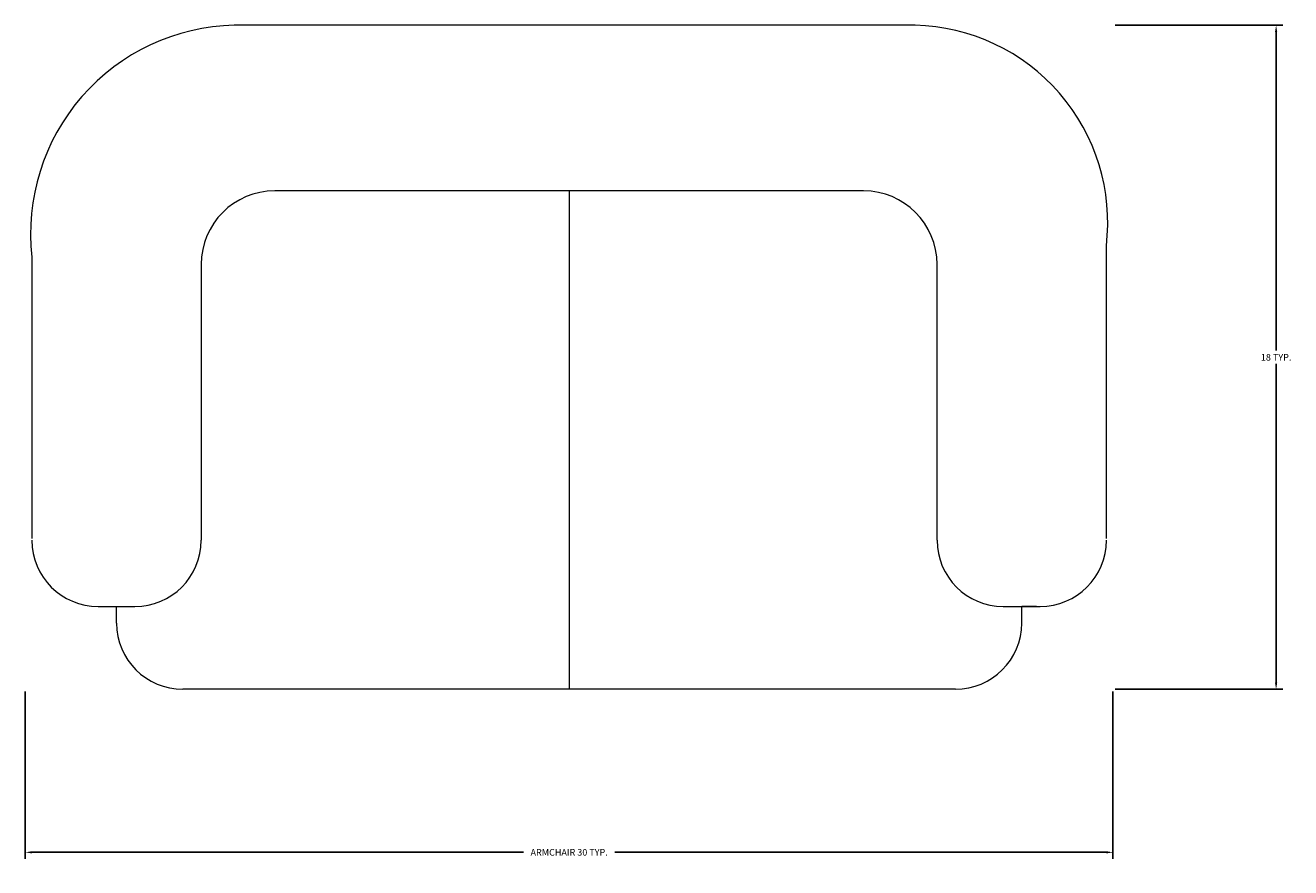
# Model space of a CAD drawing. Units: inches. Extents: x 2070 to 4408, y 1595 to 4269.
# Tile 19 of 20: x 4374 to 4408, y 3683 to 3705. Entities that reach past the tile are written whole.
import ezdxf

# ---------------------------------------------------------------- set-up
doc = ezdxf.new("R2010")
doc.units = ezdxf.units.IN
doc.layers.add('A-ANNO-DIMS', color=2, linetype='Continuous', lineweight=18)
doc.layers.add('A-FURN', color=8, linetype='Continuous', lineweight=18)
doc.styles.get("Standard").update_dxf_attribs({"font": 'arial.ttf'})
doc.dimstyles.get("Standard").update_dxf_attribs({"dimtxt": 0.18, "dimasz": 0.18, "dimexe": 0.18, "dimexo": 0.0625, "dimgap": 0.09, "dimtad": 0, "dimtih": 1, "dimtoh": 1, "dimdec": 4, "dimzin": 0, "dimdsep": 46, "dimtxsty": 'Standard', "dimcen": 0.09, "dimadec": 0, "dimazin": 0, "dimtfac": 1, "dimtdec": 4, "dimtofl": 0, "dimtmove": 0, "dimatfit": 3, "dimfxl": 1, "dimtolj": 1, "dimtzin": 0, "dimarcsym": 0})

# ---------------------------------------------------------------- blocks, each defined once
blk = doc.blocks.new('A$C6D011943')
for p, q in [((1.4484, 1.0893), (0.3319, 1.0893)), ((1.3639, 0.8177), (0.3983, 0.8177)), ((0.8811, 0.8177), (0.8811, 0)), ((1.7622, 0.2474), (1.7622, 0.7272)), ((0, 0.7091), (0, 0.2474)), ((0.2776, 0.697), (0.2776, 0.2444)), ((1.4846, 0.2444), (1.4846, 0.697)), ((0.1086, 0.1358), (0.169, 0.1358)), ((0.1388, 0.1086), (0.1388, 0.1358)), ((1.5932, 0.1358), (1.6536, 0.1358)), ((1.6475, 0.1358), (1.6234, 0.1358)), ((1.6234, 0.1086), (1.6234, 0.1358)), ((1.5148, 0), (0.2474, 0))]:
    blk.add_line(p, q)
for centre, radius, start, end in [((0.3394, 0.7478), 0.3416, 91.2564, 186.501), ((1.4409, 0.7658), 0.3236, 353.159, 88.6697), ((0.3983, 0.697), 0.1207, 90, 180), ((1.3639, 0.697), 0.1207, 0, 90), ((0.1086, 0.2444), 0.1086, 180, 270), ((0.169, 0.2444), 0.1086, 270, 0), ((1.5932, 0.2444), 0.1086, 180, 270), ((1.6536, 0.2444), 0.1086, 270, 0), ((0.2474, 0.1086), 0.1086, 180, 270), ((1.5148, 0.1086), 0.1086, 270, 0)]:
    blk.add_arc(centre, radius, start, end)
blk = doc.blocks.new('*D13')
at = {"layer": 'A-ANNO-DIMS', "color": 0, "lineweight": -2, "transparency": 16777216}
for p, q in [((4373.672, 3687.341), (4373.672, 3682.785)), ((4403.261, 3687.341), (4403.261, 3682.785)), ((4373.852, 3682.965), (4387.228, 3682.965)), ((4403.081, 3682.965), (4389.706, 3682.965))]:
    blk.add_line(p, q, dxfattribs=at)
at = {"layer": 'A-ANNO-DIMS', "color": 0, "transparency": 16777216}
for points in [[(4373.852, 3682.995), (4373.852, 3682.935), (4373.672, 3682.965)], [(4403.081, 3682.995), (4403.081, 3682.935), (4403.261, 3682.965)]]:
    blk.add_solid(points, dxfattribs=at)
at = {"layer": 'Defpoints', "color": 0, "transparency": 16777216}
for p in [(4373.672, 3687.403), (4403.261, 3687.403), (4403.261, 3682.965)]:
    blk.add_point(p, dxfattribs=at)
at = {"layer": 'A-ANNO-DIMS', "color": 0, "transparency": 16777216, "insert": (4388.467, 3682.965), "char_height": 0.18, "attachment_point": 5}
blk.add_mtext('\\A1;ARMCHAIR 30 TYP.', dxfattribs=at)
blk = doc.blocks.new('*D14')
at = {"layer": 'A-ANNO-DIMS', "color": 0, "lineweight": -2, "transparency": 16777216}
for p, q in [((4403.324, 3705.471), (4407.879, 3705.471)), ((4407.699, 3705.291), (4407.699, 3696.619)), ((4407.699, 3687.583), (4407.699, 3696.255)), ((4403.324, 3687.403), (4407.879, 3687.403))]:
    blk.add_line(p, q, dxfattribs=at)
at = {"layer": 'A-ANNO-DIMS', "color": 0, "transparency": 16777216}
for points in [[(4407.669, 3705.291), (4407.729, 3705.291), (4407.699, 3705.471)], [(4407.669, 3687.583), (4407.729, 3687.583), (4407.699, 3687.403)]]:
    blk.add_solid(points, dxfattribs=at)
at = {"layer": 'Defpoints', "color": 0, "transparency": 16777216}
for p in [(4403.261, 3705.471), (4407.699, 3705.471), (4403.261, 3687.403)]:
    blk.add_point(p, dxfattribs=at)
at = {"layer": 'A-ANNO-DIMS', "color": 0, "transparency": 16777216, "insert": (4407.699, 3696.437), "char_height": 0.18, "attachment_point": 5}
blk.add_mtext('\\A1;18 TYP.', dxfattribs=at)

msp = doc.modelspace()

# ---------------------------------------------------------------- block references
at = {"layer": 'A-FURN', "xscale": 16.58622898764873, "yscale": 16.58622898764873, "zscale": 16.58622898764873}
msp.add_blockref('A$C6D011943', (4373.8527, 3687.4033), dxfattribs=at)

# ---------------------------------------------------------------- dimensions: what is measured, and where the dimension line sits
at = {"layer": 'A-ANNO-DIMS'}
dim = msp.add_linear_dim(base=(4407.6995, 3705.4709), p1=(4403.2611, 3687.4033), p2=(4403.2611, 3705.4709), angle=90, text='<> TYP.', dimstyle='Standard', override={"dimdec": 0, "dimlfac": 1, "dimrnd": 0, "dimzin": 0, "dimdsep": 46, "dimlunit": 2}, dxfattribs=at)
dim.commit()
dim.dimension.update_dxf_attribs({"geometry": '*D14', "text_midpoint": (4407.6995, 3696.4371)})
dim = msp.add_linear_dim(base=(4403.2611, 3682.965), p1=(4373.6724, 3687.4033), p2=(4403.2611, 3687.4033), text='ARMCHAIR <> TYP.', dimstyle='Standard', override={"dimdec": 0, "dimlfac": 1, "dimrnd": 0, "dimzin": 0, "dimdsep": 46, "dimlunit": 2}, dxfattribs=at)
dim.commit()
dim.dimension.update_dxf_attribs({"geometry": '*D13', "text_midpoint": (4388.4668, 3682.965)})

doc.saveas('drawing.dxf')
